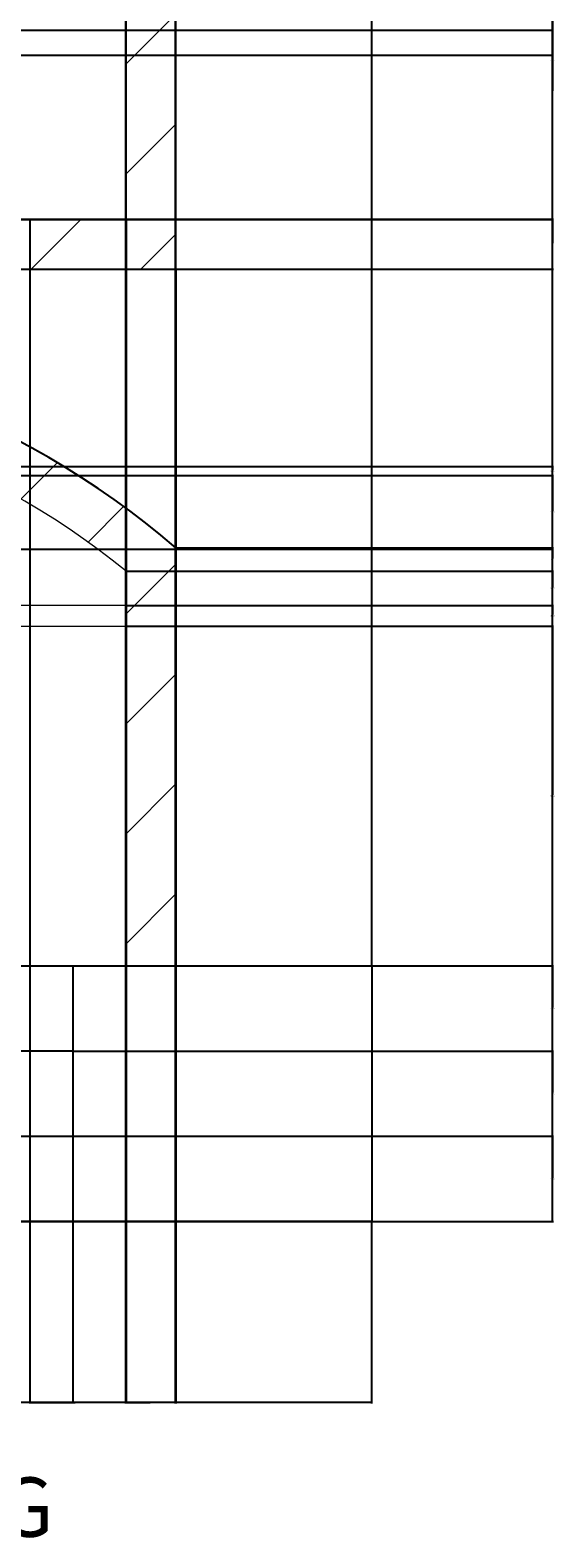
# Model space of a CAD drawing. Units: inches. Extents: x -14 to 375, y -86 to 549.
# Tile 5 of 12: x 290 to 375, y -86 to 156. Entities that reach past the tile are written whole.
import ezdxf

# ---------------------------------------------------------------- set-up
doc = ezdxf.new("R2010")
doc.units = ezdxf.units.IN
doc.header["$MEASUREMENT"] = 0
for name, color, linetype, lineweight in [('A-ANNO-DIMS', 2, 'Continuous', 18), ('A-ANNO-TEXT', 7, 'Continuous', 25), ('A-ELEV', 7, 'Continuous', 25), ('A-ELEV-PATT', 8, 'Continuous', 13), ('A-GLAZ', 4, 'Continuous', 18)]:
    doc.layers.add(name, color=color, linetype=linetype, lineweight=lineweight)
doc.styles.get("Standard").update_dxf_attribs({"font": 'arial.ttf'})
doc.dimstyles.get("Standard").update_dxf_attribs({"dimtxt": 0.18, "dimasz": 0.18, "dimexe": 0.18, "dimexo": 0.0625, "dimgap": 0.09, "dimtad": 0, "dimtih": 1, "dimtoh": 1, "dimdec": 4, "dimzin": 0, "dimdsep": 46, "dimtxsty": 'Standard', "dimcen": 0.09, "dimadec": 0, "dimazin": 0, "dimtfac": 1, "dimtdec": 4, "dimtofl": 0, "dimtmove": 0, "dimatfit": 3, "dimfxl": 1, "dimtolj": 1, "dimtzin": 0, "dimarcsym": 0})

# ---------------------------------------------------------------- blocks, each defined once
blk = doc.blocks.new('*D4')
at = {"layer": 'A-ANNO-DIMS', "color": 0, "lineweight": -2, "transparency": 16777216}
for p, q in [((15.4, -35.17), (15.4, -64.39)), ((345.26, -35.17), (345.26, -64.39)), ((15.58, -64.21), (179.87, -64.21)), ((345.08, -64.21), (180.8, -64.21))]:
    blk.add_line(p, q, dxfattribs=at)
at = {"layer": 'A-ANNO-DIMS', "color": 0, "transparency": 16777216}
for points in [[(15.58, -64.18), (15.58, -64.24), (15.4, -64.21)], [(345.08, -64.18), (345.08, -64.24), (345.26, -64.21)]]:
    blk.add_solid(points, dxfattribs=at)
at = {"layer": 'Defpoints', "color": 0, "transparency": 16777216}
for p in [(15.4, -35.11), (345.26, -35.11), (345.26, -64.21)]:
    blk.add_point(p, dxfattribs=at)
at = {"layer": 'A-ANNO-DIMS', "color": 0, "transparency": 16777216, "insert": (180.33, -64.21), "char_height": 0.18, "attachment_point": 5}
blk.add_mtext('\\A1;329.86', dxfattribs=at)
blk = doc.blocks.new('*D10')
at = {"layer": 'A-ANNO-DIMS', "color": 0, "lineweight": -2, "transparency": 16777216}
for p, q in [((301.52, 485.96), (374.54, 485.96)), ((374.36, 485.78), (374.36, 225.61)), ((374.36, -34.93), (374.36, 225.24)), ((345.33, -35.11), (374.54, -35.11))]:
    blk.add_line(p, q, dxfattribs=at)
at = {"layer": 'A-ANNO-DIMS', "color": 0, "transparency": 16777216}
for points in [[(374.33, 485.78), (374.39, 485.78), (374.36, 485.96)], [(374.33, -34.93), (374.39, -34.93), (374.36, -35.11)]]:
    blk.add_solid(points, dxfattribs=at)
at = {"layer": 'Defpoints', "color": 0, "transparency": 16777216}
for p in [(301.46, 485.96), (374.36, 485.96), (345.26, -35.11)]:
    blk.add_point(p, dxfattribs=at)
at = {"layer": 'A-ANNO-DIMS', "color": 0, "transparency": 16777216, "insert": (374.36, 225.42), "char_height": 0.18, "attachment_point": 5}
blk.add_mtext('\\A1;521.1', dxfattribs=at)
blk = doc.blocks.new('*D28')
at = {"layer": 'A-ANNO-DIMS', "color": 0, "lineweight": -2, "transparency": 16777216}
for p, q in [((107.764387, 156.376775), (374.544714, 156.376775)), ((374.364714, 156.196775), (374.364714, 154.556775)), ((374.364714, 152.556775), (374.364714, 154.196775)), ((111.764387, 152.376775), (374.544714, 152.376775))]:
    blk.add_line(p, q, dxfattribs=at)
at = {"layer": 'A-ANNO-DIMS', "color": 0, "transparency": 16777216}
for points in [[(374.334714, 156.196775), (374.394714, 156.196775), (374.364714, 156.376775)], [(374.334714, 152.556775), (374.394714, 152.556775), (374.364714, 152.376775)]]:
    blk.add_solid(points, dxfattribs=at)
at = {"layer": 'Defpoints', "color": 0, "transparency": 16777216}
for p in [(107.701887, 156.376775), (374.364714, 156.376775), (111.701887, 152.376775)]:
    blk.add_point(p, dxfattribs=at)
at = {"layer": 'A-ANNO-DIMS', "color": 0, "transparency": 16777216, "insert": (374.364714, 154.376775), "char_height": 0.18, "attachment_point": 5}
blk.add_mtext('\\A1;4', dxfattribs=at)
blk = doc.blocks.new('*D29')
at = {"layer": 'A-ANNO-DIMS', "color": 0, "lineweight": -2, "transparency": 16777216}
for p, q in [((107.74, 193.48), (374.54, 193.48)), ((374.36, 193.3), (374.36, 175.11)), ((374.36, 156.56), (374.36, 174.75)), ((107.76, 156.38), (374.54, 156.38))]:
    blk.add_line(p, q, dxfattribs=at)
at = {"layer": 'A-ANNO-DIMS', "color": 0, "transparency": 16777216}
for points in [[(374.33, 193.3), (374.39, 193.3), (374.36, 193.48)], [(374.33, 156.56), (374.39, 156.56), (374.36, 156.38)]]:
    blk.add_solid(points, dxfattribs=at)
at = {"layer": 'Defpoints', "color": 0, "transparency": 16777216}
for p in [(107.68, 193.48), (374.36, 193.48), (107.7, 156.38)]:
    blk.add_point(p, dxfattribs=at)
at = {"layer": 'A-ANNO-DIMS', "color": 0, "transparency": 16777216, "insert": (374.36, 174.93), "char_height": 0.18, "attachment_point": 5}
blk.add_mtext('\\A1;37.106', dxfattribs=at)
blk = doc.blocks.new('*D43')
at = {"layer": 'A-ANNO-DIMS', "color": 0, "lineweight": -2, "transparency": 16777216}
for p, q in [((142.23, 270.64), (142.23, -64.39)), ((305.63, 270.64), (305.63, -64.39)), ((142.41, -64.21), (223.55, -64.21)), ((305.45, -64.21), (224.32, -64.21))]:
    blk.add_line(p, q, dxfattribs=at)
at = {"layer": 'A-ANNO-DIMS', "color": 0, "transparency": 16777216}
for points in [[(142.41, -64.18), (142.41, -64.24), (142.23, -64.21)], [(305.45, -64.18), (305.45, -64.24), (305.63, -64.21)]]:
    blk.add_solid(points, dxfattribs=at)
at = {"layer": 'Defpoints', "color": 0, "transparency": 16777216}
for p in [(142.23, 270.71), (305.63, 270.71), (305.63, -64.21)]:
    blk.add_point(p, dxfattribs=at)
at = {"layer": 'A-ANNO-DIMS', "color": 0, "transparency": 16777216, "insert": (223.93, -64.21), "char_height": 0.18, "attachment_point": 5}
blk.add_mtext('\\A1;163.4', dxfattribs=at)
blk = doc.blocks.new('*D44')
at = {"layer": 'A-ANNO-DIMS', "color": 0, "lineweight": -2, "transparency": 16777216}
for p, q in [((305.63, 270.64), (305.63, -64.39)), ((313.63, 262.64), (313.63, -64.39)), ((305.81, -64.21), (309.48, -64.21)), ((313.45, -64.21), (309.78, -64.21))]:
    blk.add_line(p, q, dxfattribs=at)
at = {"layer": 'A-ANNO-DIMS', "color": 0, "transparency": 16777216}
for points in [[(305.81, -64.18), (305.81, -64.24), (305.63, -64.21)], [(313.45, -64.18), (313.45, -64.24), (313.63, -64.21)]]:
    blk.add_solid(points, dxfattribs=at)
at = {"layer": 'Defpoints', "color": 0, "transparency": 16777216}
for p in [(305.63, 270.71), (313.63, 262.71), (313.63, -64.21)]:
    blk.add_point(p, dxfattribs=at)
at = {"layer": 'A-ANNO-DIMS', "color": 0, "transparency": 16777216, "insert": (309.63, -64.21), "char_height": 0.18, "attachment_point": 5}
blk.add_mtext('\\A1;8', dxfattribs=at)
blk = doc.blocks.new('*D73')
at = {"layer": 'A-ANNO-DIMS', "color": 0, "lineweight": -2, "transparency": 16777216}
for p, q in [((234.47, 166.97), (374.54, 166.97)), ((374.36, 166.79), (374.36, 146.65)), ((374.36, 126.15), (374.36, 146.29)), ((269.47, 125.97), (374.54, 125.97))]:
    blk.add_line(p, q, dxfattribs=at)
at = {"layer": 'A-ANNO-DIMS', "color": 0, "transparency": 16777216}
for points in [[(374.33, 166.79), (374.39, 166.79), (374.36, 166.97)], [(374.33, 126.15), (374.39, 126.15), (374.36, 125.97)]]:
    blk.add_solid(points, dxfattribs=at)
at = {"layer": 'Defpoints', "color": 0, "transparency": 16777216}
for p in [(234.41, 166.97), (374.36, 166.97), (269.41, 125.97)]:
    blk.add_point(p, dxfattribs=at)
at = {"layer": 'A-ANNO-DIMS', "color": 0, "transparency": 16777216, "insert": (374.36, 146.47), "char_height": 0.18, "attachment_point": 5}
blk.add_mtext('\\A1;41', dxfattribs=at)
blk = doc.blocks.new('*D83')
at = {"layer": 'A-ANNO-DIMS', "color": 0, "lineweight": -2, "transparency": 16777216}
for p, q in [((290.24, 125.9), (290.24, -64.39)), ((305.77, 125.9), (305.77, -64.39)), ((290.42, -64.21), (297.55, -64.21)), ((305.59, -64.21), (298.46, -64.21))]:
    blk.add_line(p, q, dxfattribs=at)
at = {"layer": 'A-ANNO-DIMS', "color": 0, "transparency": 16777216}
for points in [[(290.42, -64.18), (290.42, -64.24), (290.24, -64.21)], [(305.59, -64.18), (305.59, -64.24), (305.77, -64.21)]]:
    blk.add_solid(points, dxfattribs=at)
at = {"layer": 'Defpoints', "color": 0, "transparency": 16777216}
for p in [(290.24, 125.96), (305.77, 125.96), (305.77, -64.21)]:
    blk.add_point(p, dxfattribs=at)
at = {"layer": 'A-ANNO-DIMS', "color": 0, "transparency": 16777216, "insert": (298, -64.21), "char_height": 0.18, "attachment_point": 5}
blk.add_mtext('\\A1;15.534', dxfattribs=at)
blk = doc.blocks.new('*D84')
at = {"layer": 'A-ANNO-DIMS', "color": 0, "lineweight": -2, "transparency": 16777216}
for p, q in [((305.77, 125.9), (305.77, -64.39)), ((313.77, 117.9), (313.77, -64.39)), ((305.95, -64.21), (309.62, -64.21)), ((313.59, -64.21), (309.92, -64.21))]:
    blk.add_line(p, q, dxfattribs=at)
at = {"layer": 'A-ANNO-DIMS', "color": 0, "transparency": 16777216}
for points in [[(305.95, -64.18), (305.95, -64.24), (305.77, -64.21)], [(313.59, -64.18), (313.59, -64.24), (313.77, -64.21)]]:
    blk.add_solid(points, dxfattribs=at)
at = {"layer": 'Defpoints', "color": 0, "transparency": 16777216}
for p in [(305.77, 125.96), (313.77, 117.96), (313.77, -64.21)]:
    blk.add_point(p, dxfattribs=at)
at = {"layer": 'A-ANNO-DIMS', "color": 0, "transparency": 16777216, "insert": (309.77, -64.21), "char_height": 0.18, "attachment_point": 5}
blk.add_mtext('\\A1;8', dxfattribs=at)
blk = doc.blocks.new('*D90')
at = {"layer": 'A-ANNO-DIMS', "color": 0, "lineweight": -2, "transparency": 16777216}
for p, q in [((305.83, 125.96), (374.54, 125.96)), ((374.36, 125.78), (374.36, 122.14)), ((374.36, 118.14), (374.36, 121.78)), ((313.83, 117.96), (374.54, 117.96))]:
    blk.add_line(p, q, dxfattribs=at)
at = {"layer": 'A-ANNO-DIMS', "color": 0, "transparency": 16777216}
for points in [[(374.33, 125.78), (374.39, 125.78), (374.36, 125.96)], [(374.33, 118.14), (374.39, 118.14), (374.36, 117.96)]]:
    blk.add_solid(points, dxfattribs=at)
at = {"layer": 'Defpoints', "color": 0, "transparency": 16777216}
for p in [(305.77, 125.96), (374.36, 125.96), (313.77, 117.96)]:
    blk.add_point(p, dxfattribs=at)
at = {"layer": 'A-ANNO-DIMS', "color": 0, "transparency": 16777216, "insert": (374.36, 121.96), "char_height": 0.18, "attachment_point": 5}
blk.add_mtext('\\A1;8', dxfattribs=at)
blk = doc.blocks.new('*D91')
at = {"layer": 'A-ANNO-DIMS', "color": 0, "lineweight": -2, "transparency": 16777216}
for p, q in [((305.83, 176.93), (374.54, 176.93)), ((374.36, 176.75), (374.36, 151.63)), ((374.36, 126.14), (374.36, 151.26)), ((305.83, 125.96), (374.54, 125.96))]:
    blk.add_line(p, q, dxfattribs=at)
at = {"layer": 'A-ANNO-DIMS', "color": 0, "transparency": 16777216}
for points in [[(374.33, 176.75), (374.39, 176.75), (374.36, 176.93)], [(374.33, 126.14), (374.39, 126.14), (374.36, 125.96)]]:
    blk.add_solid(points, dxfattribs=at)
at = {"layer": 'Defpoints', "color": 0, "transparency": 16777216}
for p in [(305.77, 176.93), (374.36, 176.93), (305.77, 125.96)]:
    blk.add_point(p, dxfattribs=at)
at = {"layer": 'A-ANNO-DIMS', "color": 0, "transparency": 16777216, "insert": (374.36, 151.45), "char_height": 0.18, "attachment_point": 5}
blk.add_mtext('\\A1;50.97', dxfattribs=at)
blk = doc.blocks.new('*D106')
at = {"layer": 'A-ANNO-DIMS', "color": 0, "lineweight": -2, "transparency": 16777216}
for p, q in [((275.19, 6.02), (275.19, 515.24)), ((275.37, 515.06), (290.01, 515.06)), ((305.59, 515.06), (290.94, 515.06)), ((305.77, 6.02), (305.77, 515.24))]:
    blk.add_line(p, q, dxfattribs=at)
at = {"layer": 'A-ANNO-DIMS', "color": 0, "transparency": 16777216}
for points in [[(275.37, 515.09), (275.37, 515.03), (275.19, 515.06)], [(305.59, 515.09), (305.59, 515.03), (305.77, 515.06)]]:
    blk.add_solid(points, dxfattribs=at)
at = {"layer": 'Defpoints', "color": 0, "transparency": 16777216}
for p in [(305.77, 515.06), (275.19, 5.96), (305.77, 5.96)]:
    blk.add_point(p, dxfattribs=at)
at = {"layer": 'A-ANNO-DIMS', "color": 0, "transparency": 16777216, "insert": (290.48, 515.06), "char_height": 0.18, "attachment_point": 5}
blk.add_mtext('\\A1;30.585', dxfattribs=at)
blk = doc.blocks.new('*D107')
at = {"layer": 'A-ANNO-DIMS', "color": 0, "lineweight": -2, "transparency": 16777216}
for p, q in [((305.77, 6.02), (305.77, 515.24)), ((305.95, 515.06), (309.62, 515.06)), ((313.59, 515.06), (309.92, 515.06)), ((313.77, 6.02), (313.77, 515.24))]:
    blk.add_line(p, q, dxfattribs=at)
at = {"layer": 'A-ANNO-DIMS', "color": 0, "transparency": 16777216}
for points in [[(305.95, 515.09), (305.95, 515.03), (305.77, 515.06)], [(313.59, 515.09), (313.59, 515.03), (313.77, 515.06)]]:
    blk.add_solid(points, dxfattribs=at)
at = {"layer": 'Defpoints', "color": 0, "transparency": 16777216}
for p in [(313.77, 515.06), (305.77, 5.96), (313.77, 5.96)]:
    blk.add_point(p, dxfattribs=at)
at = {"layer": 'A-ANNO-DIMS', "color": 0, "transparency": 16777216, "insert": (309.77, 515.06), "char_height": 0.18, "attachment_point": 5}
blk.add_mtext('\\A1;8', dxfattribs=at)
blk = doc.blocks.new('*D109')
at = {"layer": 'A-ANNO-DIMS', "color": 0, "lineweight": -2, "transparency": 16777216}
for p, q in [((152.96, -7.79), (152.96, -64.39)), ((297.19, -7.79), (297.19, -64.39)), ((153.14, -64.21), (224.62, -64.21)), ((297.01, -64.21), (225.53, -64.21))]:
    blk.add_line(p, q, dxfattribs=at)
at = {"layer": 'A-ANNO-DIMS', "color": 0, "transparency": 16777216}
for points in [[(153.14, -64.18), (153.14, -64.24), (152.96, -64.21)], [(297.01, -64.18), (297.01, -64.24), (297.19, -64.21)]]:
    blk.add_solid(points, dxfattribs=at)
at = {"layer": 'Defpoints', "color": 0, "transparency": 16777216}
for p in [(152.96, -7.73), (297.19, -7.73), (297.19, -64.21)]:
    blk.add_point(p, dxfattribs=at)
at = {"layer": 'A-ANNO-DIMS', "color": 0, "transparency": 16777216, "insert": (225.08, -64.21), "char_height": 0.18, "attachment_point": 5}
blk.add_mtext('\\A1;144.23', dxfattribs=at)
blk = doc.blocks.new('*D112')
at = {"layer": 'A-ANNO-DIMS', "color": 0, "lineweight": -2, "transparency": 16777216}
for p, q in [((297.26, 5.96), (374.54, 5.96)), ((374.36, 5.78), (374.36, -0.7)), ((374.36, -7.55), (374.36, -1.07)), ((297.26, -7.73), (374.54, -7.73))]:
    blk.add_line(p, q, dxfattribs=at)
at = {"layer": 'A-ANNO-DIMS', "color": 0, "transparency": 16777216}
for points in [[(374.33, 5.78), (374.39, 5.78), (374.36, 5.96)], [(374.33, -7.55), (374.39, -7.55), (374.36, -7.73)]]:
    blk.add_solid(points, dxfattribs=at)
at = {"layer": 'Defpoints', "color": 0, "transparency": 16777216}
for p in [(297.19, 5.96), (297.19, -7.73), (374.36, -7.73)]:
    blk.add_point(p, dxfattribs=at)
at = {"layer": 'A-ANNO-DIMS', "color": 0, "transparency": 16777216, "insert": (374.36, -0.89), "char_height": 0.18, "attachment_point": 5}
blk.add_mtext('\\A1;13.69', dxfattribs=at)
blk = doc.blocks.new('*D113')
at = {"layer": 'A-ANNO-DIMS', "color": 0, "lineweight": -2, "transparency": 16777216}
for p, q in [((297.26, -7.73), (374.54, -7.73)), ((374.36, -7.91), (374.36, -14.39)), ((374.36, -21.24), (374.36, -14.76)), ((274.26, -21.42), (374.54, -21.42))]:
    blk.add_line(p, q, dxfattribs=at)
at = {"layer": 'A-ANNO-DIMS', "color": 0, "transparency": 16777216}
for points in [[(374.33, -7.91), (374.39, -7.91), (374.36, -7.73)], [(374.33, -21.24), (374.39, -21.24), (374.36, -21.42)]]:
    blk.add_solid(points, dxfattribs=at)
at = {"layer": 'Defpoints', "color": 0, "transparency": 16777216}
for p in [(297.19, -7.73), (274.19, -21.42), (374.36, -21.42)]:
    blk.add_point(p, dxfattribs=at)
at = {"layer": 'A-ANNO-DIMS', "color": 0, "transparency": 16777216, "insert": (374.36, -14.58), "char_height": 0.18, "attachment_point": 5}
blk.add_mtext('\\A1;13.69', dxfattribs=at)
blk = doc.blocks.new('*D114')
at = {"layer": 'A-ANNO-DIMS', "color": 0, "lineweight": -2, "transparency": 16777216}
for p, q in [((274.26, -21.42), (374.54, -21.42)), ((374.36, -21.6), (374.36, -28.08)), ((374.36, -34.93), (374.36, -28.45)), ((262.26, -35.11), (374.54, -35.11))]:
    blk.add_line(p, q, dxfattribs=at)
at = {"layer": 'A-ANNO-DIMS', "color": 0, "transparency": 16777216}
for points in [[(374.33, -21.6), (374.39, -21.6), (374.36, -21.42)], [(374.33, -34.93), (374.39, -34.93), (374.36, -35.11)]]:
    blk.add_solid(points, dxfattribs=at)
at = {"layer": 'Defpoints', "color": 0, "transparency": 16777216}
for p in [(274.19, -21.42), (262.19, -35.11), (374.36, -35.11)]:
    blk.add_point(p, dxfattribs=at)
at = {"layer": 'A-ANNO-DIMS', "color": 0, "transparency": 16777216, "insert": (374.36, -28.27), "char_height": 0.18, "attachment_point": 5}
blk.add_mtext('\\A1;13.69', dxfattribs=at)
blk = doc.blocks.new('*D115')
at = {"layer": 'A-ANNO-DIMS', "color": 0, "lineweight": -2, "transparency": 16777216}
for p, q in [((305.83, 60.59), (374.54, 60.59)), ((374.36, 60.41), (374.36, 33.46)), ((374.36, 6.14), (374.36, 33.09)), ((313.83, 5.96), (374.54, 5.96))]:
    blk.add_line(p, q, dxfattribs=at)
at = {"layer": 'A-ANNO-DIMS', "color": 0, "transparency": 16777216}
for points in [[(374.33, 60.41), (374.39, 60.41), (374.36, 60.59)], [(374.33, 6.14), (374.39, 6.14), (374.36, 5.96)]]:
    blk.add_solid(points, dxfattribs=at)
at = {"layer": 'Defpoints', "color": 0, "transparency": 16777216}
for p in [(305.77, 60.59), (374.36, 60.59), (313.77, 5.96)]:
    blk.add_point(p, dxfattribs=at)
at = {"layer": 'A-ANNO-DIMS', "color": 0, "transparency": 16777216, "insert": (374.36, 33.27), "char_height": 0.18, "attachment_point": 5}
blk.add_mtext('\\A1;54.63', dxfattribs=at)
blk = doc.blocks.new('*D116')
at = {"layer": 'A-ANNO-DIMS', "color": 0, "lineweight": -2, "transparency": 16777216}
for p, q in [((305.83, 63.92), (374.54, 63.92)), ((374.36, 63.74), (374.36, 62.44)), ((305.83, 60.59), (374.54, 60.59)), ((374.36, 60.77), (374.36, 62.07))]:
    blk.add_line(p, q, dxfattribs=at)
at = {"layer": 'A-ANNO-DIMS', "color": 0, "transparency": 16777216}
for points in [[(374.33, 63.74), (374.39, 63.74), (374.36, 63.92)], [(374.33, 60.77), (374.39, 60.77), (374.36, 60.59)]]:
    blk.add_solid(points, dxfattribs=at)
at = {"layer": 'Defpoints', "color": 0, "transparency": 16777216}
for p in [(305.77, 63.92), (374.36, 63.92), (305.77, 60.59)]:
    blk.add_point(p, dxfattribs=at)
at = {"layer": 'A-ANNO-DIMS', "color": 0, "transparency": 16777216, "insert": (374.36, 62.26), "char_height": 0.18, "attachment_point": 5}
blk.add_mtext('\\A1;3.333', dxfattribs=at)
blk = doc.blocks.new('*D117')
at = {"layer": 'A-ANNO-DIMS', "color": 0, "lineweight": -2, "transparency": 16777216}
for p, q in [((305.83, 69.42), (374.54, 69.42)), ((374.36, 69.24), (374.36, 66.85)), ((374.36, 64.1), (374.36, 66.49)), ((305.83, 63.92), (374.54, 63.92))]:
    blk.add_line(p, q, dxfattribs=at)
at = {"layer": 'A-ANNO-DIMS', "color": 0, "transparency": 16777216}
for points in [[(374.33, 69.24), (374.39, 69.24), (374.36, 69.42)], [(374.33, 64.1), (374.39, 64.1), (374.36, 63.92)]]:
    blk.add_solid(points, dxfattribs=at)
at = {"layer": 'Defpoints', "color": 0, "transparency": 16777216}
for p in [(305.77, 69.42), (374.36, 69.42), (305.77, 63.92)]:
    blk.add_point(p, dxfattribs=at)
at = {"layer": 'A-ANNO-DIMS', "color": 0, "transparency": 16777216, "insert": (374.36, 66.67), "char_height": 0.18, "attachment_point": 5}
blk.add_mtext('\\A1;5.499', dxfattribs=at)
blk = doc.blocks.new('*D118')
at = {"layer": 'A-ANNO-DIMS', "color": 0, "lineweight": -2, "transparency": 16777216}
for p, q in [((313.83, 73.17), (374.54, 73.17)), ((374.36, 72.99), (374.36, 71.48)), ((374.36, 69.6), (374.36, 71.11)), ((305.83, 69.42), (374.54, 69.42))]:
    blk.add_line(p, q, dxfattribs=at)
at = {"layer": 'A-ANNO-DIMS', "color": 0, "transparency": 16777216}
for points in [[(374.33, 72.99), (374.39, 72.99), (374.36, 73.17)], [(374.33, 69.6), (374.39, 69.6), (374.36, 69.42)]]:
    blk.add_solid(points, dxfattribs=at)
at = {"layer": 'Defpoints', "color": 0, "transparency": 16777216}
for p in [(313.77, 73.17), (374.36, 73.17), (305.77, 69.42)]:
    blk.add_point(p, dxfattribs=at)
at = {"layer": 'A-ANNO-DIMS', "color": 0, "transparency": 16777216, "insert": (374.36, 71.3), "char_height": 0.18, "attachment_point": 5}
blk.add_mtext('\\A1;3.751', dxfattribs=at)
blk = doc.blocks.new('*D128')
at = {"layer": 'A-ANNO-DIMS', "color": 0, "lineweight": -2, "transparency": 16777216}
for p, q in [((96.79, 84.82), (374.54, 84.82)), ((374.36, 84.64), (374.36, 79.07)), ((374.36, 73.15), (374.36, 78.71)), ((111.56, 72.97), (374.54, 72.97))]:
    blk.add_line(p, q, dxfattribs=at)
at = {"layer": 'A-ANNO-DIMS', "color": 0, "transparency": 16777216}
for points in [[(374.33, 84.64), (374.39, 84.64), (374.36, 84.82)], [(374.33, 73.15), (374.39, 73.15), (374.36, 72.97)]]:
    blk.add_solid(points, dxfattribs=at)
at = {"layer": 'Defpoints', "color": 0, "transparency": 16777216}
for p in [(96.73, 84.82), (374.36, 84.82), (111.5, 72.97)]:
    blk.add_point(p, dxfattribs=at)
at = {"layer": 'A-ANNO-DIMS', "color": 0, "transparency": 16777216, "insert": (374.36, 78.89), "char_height": 0.18, "attachment_point": 5}
blk.add_mtext('\\A1;11.849', dxfattribs=at)
blk = doc.blocks.new('*D129')
at = {"layer": 'A-ANNO-DIMS', "color": 0, "lineweight": -2, "transparency": 16777216}
for p, q in [((96.79, 86.23), (374.54, 86.23)), ((374.36, 86.05), (374.36, 85.7)), ((374.36, 85), (374.36, 85.34)), ((96.79, 84.82), (374.54, 84.82))]:
    blk.add_line(p, q, dxfattribs=at)
at = {"layer": 'A-ANNO-DIMS', "color": 0, "transparency": 16777216}
for points in [[(374.33, 86.05), (374.39, 86.05), (374.36, 86.23)], [(374.33, 85), (374.39, 85), (374.36, 84.82)]]:
    blk.add_solid(points, dxfattribs=at)
at = {"layer": 'Defpoints', "color": 0, "transparency": 16777216}
for p in [(96.73, 86.23), (374.36, 86.23), (96.73, 84.82)]:
    blk.add_point(p, dxfattribs=at)
at = {"layer": 'A-ANNO-DIMS', "color": 0, "transparency": 16777216, "insert": (374.36, 85.52), "char_height": 0.18, "attachment_point": 5}
blk.add_mtext('\\A1;1.409', dxfattribs=at)

msp = doc.modelspace()

# ---------------------------------------------------------------- hatches: boundary and pattern name
at = {"layer": 'A-ELEV-PATT'}
h = msp.add_hatch(dxfattribs=at)
h.set_pattern_fill('ANSI31', color=256, scale=100)
h.set_pattern_definition([(45, (-168.406, -22.703), (-8.83883, 8.83883), [])])
h.paths.add_polyline_path([(313.6281, 262.7071), (313.6281, 357.9589), (313.7701, 357.9589), (313.7701, 433.1717, 0.36940998), (134.2334, 433.1717), (134.2334, 365.9589), (134.2334, 262.7071)])
h.paths.add_polyline_path([(142.2334, 270.7071), (142.2334, 365.9589), (142.2334, 429.4208, -0.35358711), (305.7701, 429.4208), (305.7701, 365.9589), (305.6281, 365.9589), (305.6281, 270.7071)], flags=16)
h.paths.add_polyline_path([(134.2334, 187.8466), (134.2334, 117.9589), (313.7701, 117.9589), (313.7701, 187.8466, 0.62486768)])
h.paths.add_polyline_path([(305.7701, 185.9589), (305.7701, 125.9589), (142.2334, 125.9589), (142.2334, 185.9589, -0.61125102)], flags=16)
h.paths.add_polyline_path([(134.2334, 73.1717), (134.2334, 5.9589), (142.2334, 5.9589), (142.2334, 69.4208, -0.35358711), (305.7701, 69.4208), (305.7701, 5.9589), (313.7701, 5.9589), (313.7701, 73.1717, 0.36940998)])

# ---------------------------------------------------------------- linework, layer by layer
at = {"layer": 'A-ELEV'}
msp.add_line((15.4018, 5.9589), (345.2647, 5.9589), dxfattribs=at)
for points in [[(345.2647, 5.9589), (345.2647, 125.9589), (345.2647, 245.9589), (345.2647, 365.9589), (345.2647, 442.1495, 0.41421356), (301.4553, 485.9589)], [(313.7701, 5.9589), (313.7701, 73.1717, 0.36940998), (134.2334, 73.1717), (134.2334, 5.9589)]]:
    msp.add_lwpolyline(points, format="xyb", dxfattribs=at)
for points in [[(134.2334, 187.8466), (134.2334, 117.9589), (313.7701, 117.9589), (313.7701, 187.8466, 0.62486768)], [(142.2334, 185.9589), (142.2334, 125.9589), (305.7701, 125.9589), (305.7701, 185.9589, 0.61125102)]]:
    msp.add_lwpolyline(points, format="xyb", close=True, dxfattribs=at)
for points in [[(15.4018, 5.9589), (345.2647, 5.9589), (345.2647, -35.1115), (15.4018, -35.1115)], [(152.9633, 5.9589), (297.193, 5.9589), (297.193, -7.7312), (152.9633, -7.7312)]]:
    msp.add_lwpolyline(points, close=True, dxfattribs=at)
at = {"layer": 'A-GLAZ'}
msp.add_lwpolyline([(305.7701, 5.9589), (305.7701, 69.4208, 0.35358711), (142.2334, 69.4208), (142.2334, 5.9589)], format="xyb", dxfattribs=at)
msp.add_lwpolyline([(275.185, 60.5886), (305.7701, 60.5886), (305.7701, 63.9218), (275.185, 63.9218)], dxfattribs=at)

# ---------------------------------------------------------------- texts
at = {"layer": 'A-ANNO-TEXT'}
msp.add_text('G+3 RESIDENTIAL BUILDING', height=9.539085, dxfattribs=at).set_placement((124.7897, -85.7919))

# ---------------------------------------------------------------- dimensions: what is measured, and where the dimension line sits
at = {"layer": 'A-ANNO-DIMS'}
for base, p1, p2, override, picture, middle in [((305.7701, 515.0589), (275.185, 5.9589), (305.7701, 5.9589), {"dimdec": 3, "dimlfac": 1, "dimrnd": 0, "dimzin": 0, "dimdsep": 46, "dimlunit": 2}, '*D106', (290.4775, 515.0589)), ((313.7701, 515.0589), (305.7701, 5.9589), (313.7701, 5.9589), {"dimdec": 0, "dimlfac": 1, "dimrnd": 0, "dimzin": 0, "dimdsep": 46, "dimlunit": 2}, '*D107', (309.7701, 515.0589)), ((305.6281, -64.2115), (142.2334, 270.7071), (305.6281, 270.7071), {"dimdec": 1, "dimlfac": 1, "dimrnd": 0, "dimzin": 0, "dimdsep": 46, "dimlunit": 2}, '*D43', (223.9307, -64.2115)), ((313.6281, -64.2115), (305.6281, 270.7071), (313.6281, 262.7071), {"dimdec": 0, "dimlfac": 1, "dimrnd": 0, "dimzin": 0, "dimdsep": 46, "dimlunit": 2}, '*D44', (309.6281, -64.2115)), ((305.77006, -64.21154), (290.23562, 125.95892), (305.77006, 125.95892), {"dimdec": 3, "dimlfac": 1, "dimrnd": 0, "dimzin": 0, "dimdsep": 46, "dimlunit": 2}, '*D83', (298.00284, -64.21154)), ((313.7701, -64.2115), (305.7701, 125.9589), (313.7701, 117.9589), {"dimdec": 0, "dimlfac": 1, "dimrnd": 0, "dimzin": 0, "dimdsep": 46, "dimlunit": 2}, '*D84', (309.7701, -64.2115)), ((297.193, -64.2115), (152.9633, -7.7312), (297.193, -7.7312), {"dimdec": 2, "dimlfac": 1, "dimrnd": 0, "dimzin": 0, "dimdsep": 46, "dimlunit": 2}, '*D109', (225.0782, -64.2115)), ((345.2647, -64.2115), (15.4018, -35.1115), (345.2647, -35.1115), {"dimdec": 2, "dimlfac": 1, "dimrnd": 0, "dimzin": 0, "dimdsep": 46, "dimlunit": 2}, '*D4', (180.3333, -64.2115))]:
    dim = msp.add_linear_dim(base=base, p1=p1, p2=p2, dimstyle='Standard', override=override, dxfattribs=at)
    dim.commit()
    dim.dimension.update_dxf_attribs({"geometry": picture, "text_midpoint": middle})
for base, p1, p2, override, picture, middle in [((374.3647, 485.9589), (345.2647, -35.1115), (301.4553, 485.9589), {"dimdec": 1, "dimlfac": 1, "dimrnd": 0, "dimzin": 0, "dimdsep": 46, "dimlunit": 2}, '*D10', (374.3647, 225.4237)), ((374.3647, 193.4825), (107.7019, 156.3768), (107.6798, 193.4825), {"dimdec": 3, "dimlfac": 1, "dimrnd": 0, "dimzin": 0, "dimdsep": 46, "dimlunit": 2}, '*D29', (374.3647, 174.9296)), ((374.3647, 176.9318), (305.7701, 125.9589), (305.7701, 176.9318), {"dimdec": 2, "dimlfac": 1, "dimrnd": 0, "dimzin": 0, "dimdsep": 46, "dimlunit": 2}, '*D91', (374.3647, 151.4454)), ((374.3647, 166.9717), (269.409, 125.9717), (234.409, 166.9717), {"dimdec": 0, "dimlfac": 1, "dimrnd": 0, "dimzin": 0, "dimdsep": 46, "dimlunit": 2}, '*D73', (374.3647, 146.4717)), ((374.3647, 156.3768), (111.7019, 152.3768), (107.7019, 156.3768), {"dimdec": 0, "dimlfac": 1, "dimrnd": 0, "dimzin": 0, "dimdsep": 46, "dimlunit": 2}, '*D28', (374.3647, 154.3768)), ((374.3647, 125.9589), (313.7701, 117.9589), (305.7701, 125.9589), {"dimdec": 0, "dimlfac": 1, "dimrnd": 0, "dimzin": 0, "dimdsep": 46, "dimlunit": 2}, '*D90', (374.3647, 121.9589)), ((374.3647, 86.2255), (96.7255, 84.8165), (96.7255, 86.2255), {"dimdec": 3, "dimlfac": 1, "dimrnd": 0, "dimzin": 0, "dimdsep": 46, "dimlunit": 2}, '*D129', (374.3647, 85.521)), ((374.3647, 84.8165), (111.4987, 72.9679), (96.7255, 84.8165), {"dimdec": 3, "dimlfac": 1, "dimrnd": 0, "dimzin": 0, "dimdsep": 46, "dimlunit": 2}, '*D128', (374.3647, 78.8922)), ((374.3647, 73.1717), (305.7701, 69.4208), (313.7701, 73.1717), {"dimdec": 3, "dimlfac": 1, "dimrnd": 0, "dimzin": 0, "dimdsep": 46, "dimlunit": 2}, '*D118', (374.3647, 71.2962)), ((374.3647, 69.4208), (305.7701, 63.9218), (305.7701, 69.4208), {"dimdec": 3, "dimlfac": 1, "dimrnd": 0, "dimzin": 0, "dimdsep": 46, "dimlunit": 2}, '*D117', (374.3647, 66.6713)), ((374.3647, 63.9218), (305.7701, 60.5886), (305.7701, 63.9218), {"dimdec": 3, "dimlfac": 1, "dimrnd": 0, "dimzin": 0, "dimdsep": 46, "dimlunit": 2}, '*D116', (374.3647, 62.2552)), ((374.3647, 60.5886), (313.7701, 5.9589), (305.7701, 60.5886), {"dimdec": 2, "dimlfac": 1, "dimrnd": 0, "dimzin": 0, "dimdsep": 46, "dimlunit": 2}, '*D115', (374.3647, 33.2738)), ((374.3647, -7.7312), (297.193, 5.9589), (297.193, -7.7312), {"dimdec": 2, "dimlfac": 1, "dimrnd": 0, "dimzin": 0, "dimdsep": 46, "dimlunit": 2}, '*D112', (374.3647, -0.8862)), ((374.3647, -21.4214), (297.193, -7.7312), (274.193, -21.4214), {"dimdec": 2, "dimlfac": 1, "dimrnd": 0, "dimzin": 0, "dimdsep": 46, "dimlunit": 2}, '*D113', (374.3647, -14.5763)), ((374.3647, -35.1115), (274.193, -21.4214), (262.193, -35.1115), {"dimdec": 2, "dimlfac": 1, "dimrnd": 0, "dimzin": 0, "dimdsep": 46, "dimlunit": 2}, '*D114', (374.3647, -28.2665))]:
    dim = msp.add_linear_dim(base=base, p1=p1, p2=p2, angle=90, dimstyle='Standard', override=override, dxfattribs=at)
    dim.commit()
    dim.dimension.update_dxf_attribs({"geometry": picture, "text_midpoint": middle})

doc.saveas('drawing.dxf')
